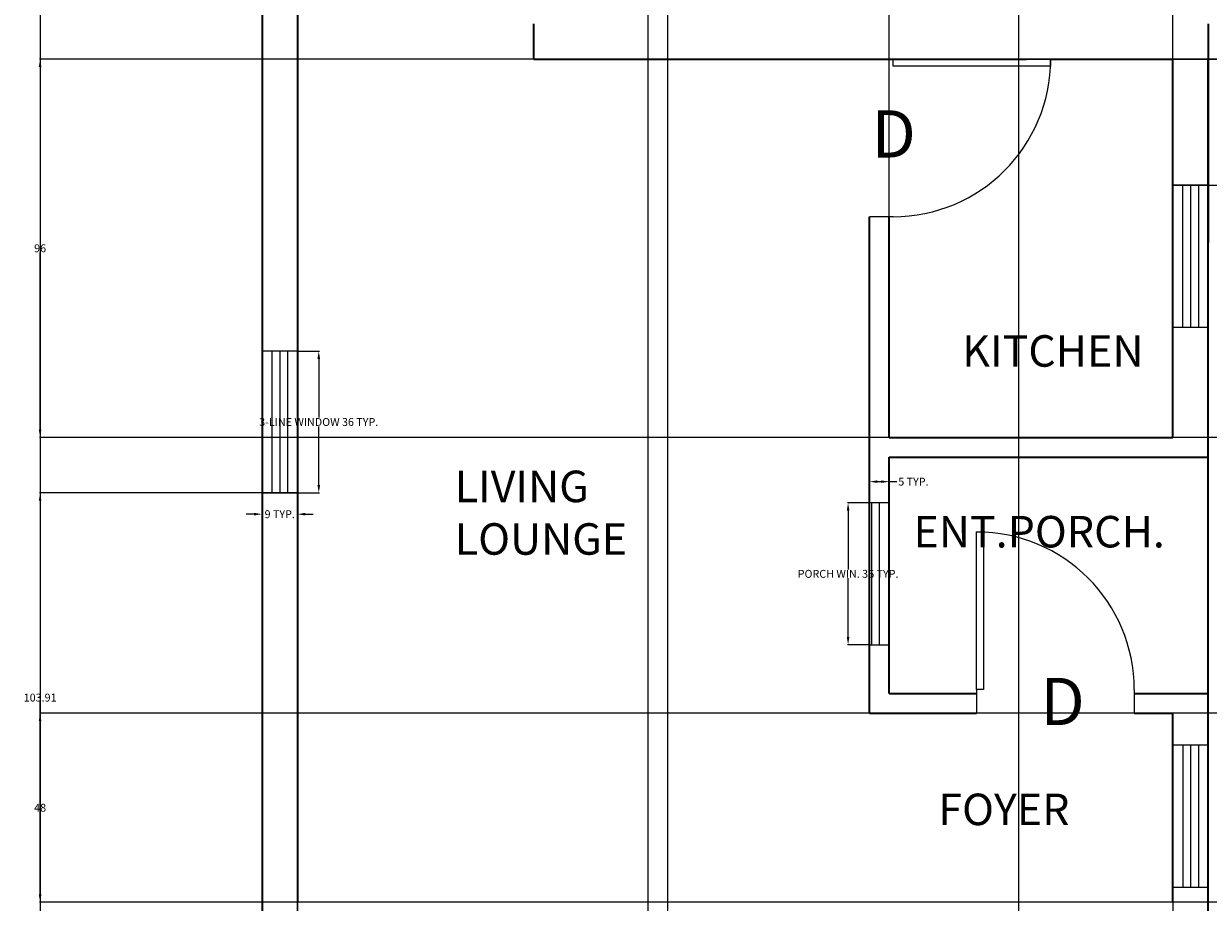
# Model space of a CAD drawing. Units: inches. Extents: x 190 to 836, y -241 to 999.
# Tile 6 of 9: x 190 to 491, y 566 to 789. Entities that reach past the tile are written whole.
import ezdxf

# ---------------------------------------------------------------- set-up
doc = ezdxf.new("R2010")
doc.units = ezdxf.units.IN
doc.header["$MEASUREMENT"] = 0
for name, color, linetype, lineweight in [('A-ANNO-DIMS', 2, 'Continuous', 18), ('A-ANNO-TEXT', 7, 'Continuous', 18), ('A-AREA-IDEN', 7, 'Continuous', 18), ('A-DOOR', 3, 'Continuous', 18), ('A-GLAZ', 4, 'Continuous', 18), ('A-WALL', 7, 'Continuous', 35)]:
    doc.layers.add(name, color=color, linetype=linetype, lineweight=lineweight)
doc.styles.get("Standard").update_dxf_attribs({"font": 'arial.ttf'})
doc.dimstyles.get("Standard").update_dxf_attribs({"dimtxt": 2, "dimasz": 2, "dimexe": 0.18, "dimexo": 0.0625, "dimgap": 0.09, "dimtad": 0, "dimtih": 1, "dimtoh": 1, "dimdec": 0, "dimzin": 0, "dimdsep": 46, "dimlunit": 3, "dimtxsty": 'Standard', "dimcen": 0.09, "dimadec": 0, "dimazin": 0, "dimtfac": 1, "dimtdec": 0, "dimtofl": 0, "dimtmove": 0, "dimatfit": 3, "dimfxl": 1, "dimtolj": 1, "dimtzin": 0, "dimarcsym": 0})

# ---------------------------------------------------------------- blocks, each defined once
blk = doc.blocks.new('*U4')
for p, q in [((-40, 0), (-40, 6)), ((0, 0), (0, 6))]:
    blk.add_line(p, q)
blk.add_lwpolyline([(0, 0), (0, -40), (-1.75, -40), (-1.75, 0)], close=True)
blk.add_arc((0, 0), 40, 180, 270)
blk = doc.blocks.new('*U5')
for p, q in [((0, 0), (0, -6)), ((40, 0), (40, -6))]:
    blk.add_line(p, q)
blk.add_lwpolyline([(0, 0), (0, 40), (1.75, 40), (1.75, 0)], close=True)
blk.add_arc((0, 0), 40, 0, 90)
blk = doc.blocks.new('WIN-36IN-9IN-3LINE')
for p, q in [((2.5, 36), (2.5, 0)), ((4.5, 36), (4.5, 0)), ((6.5, 36), (6.5, 0))]:
    blk.add_line(p, q)
blk.add_lwpolyline([(0, 0), (9, 0), (9, 36), (0, 36)], close=True)
blk = doc.blocks.new('WIN-36IN-5IN-PARTITION')
for p, q in [((5, 36), (0, 36)), ((0.5, 36), (0.5, 0)), ((2.5, 36), (2.5, 0)), ((5, 0), (5, 36)), ((0, 0), (5, 0))]:
    blk.add_line(p, q)
blk = doc.blocks.new('*D10')
at = {"layer": 'A-ANNO-DIMS', "color": 0, "lineweight": -2, "transparency": 16777216}
for p, q in [((259.5, 705.44), (265.02, 705.44)), ((264.84, 703.44), (264.84, 688.57)), ((264.84, 671.44), (264.84, 686.32)), ((259.5, 669.44), (265.02, 669.44))]:
    blk.add_line(p, q, dxfattribs=at)
at = {"layer": 'A-ANNO-DIMS', "color": 0, "transparency": 16777216}
for points in [[(264.51, 703.44), (265.18, 703.44), (264.84, 705.44)], [(264.51, 671.44), (265.18, 671.44), (264.84, 669.44)]]:
    blk.add_solid(points, dxfattribs=at)
at = {"layer": 'Defpoints', "color": 0, "transparency": 16777216}
for p in [(259.44, 705.44), (264.84, 705.44), (259.44, 669.44)]:
    blk.add_point(p, dxfattribs=at)
at = {"layer": 'A-ANNO-DIMS', "color": 0, "transparency": 16777216, "insert": (264.84, 687.44), "char_height": 2, "attachment_point": 5}
blk.add_mtext('\\A1;3-LINE WINDOW 36 TYP.', dxfattribs=at)
blk = doc.blocks.new('*D11')
at = {"layer": 'A-ANNO-DIMS', "color": 0, "lineweight": -2, "transparency": 16777216}
for p, q in [((250.44, 669.38), (250.44, 663.86)), ((259.44, 669.38), (259.44, 663.86)), ((248.44, 664.04), (246.44, 664.04)), ((261.44, 664.04), (263.44, 664.04))]:
    blk.add_line(p, q, dxfattribs=at)
at = {"layer": 'A-ANNO-DIMS', "color": 0, "transparency": 16777216}
for points in [[(248.44, 664.38), (248.44, 663.71), (250.44, 664.04)], [(261.44, 664.38), (261.44, 663.71), (259.44, 664.04)]]:
    blk.add_solid(points, dxfattribs=at)
at = {"layer": 'Defpoints', "color": 0, "transparency": 16777216}
for p in [(250.44, 669.44), (259.44, 669.44), (259.44, 664.04)]:
    blk.add_point(p, dxfattribs=at)
at = {"layer": 'A-ANNO-DIMS', "color": 0, "transparency": 16777216, "insert": (254.94, 664.04), "char_height": 2, "attachment_point": 5}
blk.add_mtext('\\A1;9 TYP.', dxfattribs=at)
blk = doc.blocks.new('*D14')
at = {"layer": 'A-ANNO-DIMS', "color": 0, "lineweight": -2, "transparency": 16777216}
for p, q in [((404.49, 666.9), (398.97, 666.9)), ((399.15, 664.9), (399.15, 650.03)), ((399.15, 632.9), (399.15, 647.77)), ((404.49, 630.9), (398.97, 630.9))]:
    blk.add_line(p, q, dxfattribs=at)
at = {"layer": 'A-ANNO-DIMS', "color": 0, "transparency": 16777216}
for points in [[(398.82, 664.9), (399.49, 664.9), (399.15, 666.9)], [(398.82, 632.9), (399.49, 632.9), (399.15, 630.9)]]:
    blk.add_solid(points, dxfattribs=at)
at = {"layer": 'Defpoints', "color": 0, "transparency": 16777216}
for p in [(399.15, 666.9), (404.55, 666.9), (404.55, 630.9)]:
    blk.add_point(p, dxfattribs=at)
at = {"layer": 'A-ANNO-DIMS', "color": 0, "transparency": 16777216, "insert": (399.15, 648.9), "char_height": 2, "attachment_point": 5}
blk.add_mtext('\\A1;PORCH WIN. 36 TYP.', dxfattribs=at)
blk = doc.blocks.new('*D15')
at = {"layer": 'A-ANNO-DIMS', "color": 0, "lineweight": -2, "transparency": 16777216}
for p, q in [((404.55, 666.96), (404.55, 672.48)), ((406.55, 672.3), (407.55, 672.3)), ((409.55, 666.96), (409.55, 672.48)), ((409.55, 672.3), (411.55, 672.3))]:
    blk.add_line(p, q, dxfattribs=at)
at = {"layer": 'A-ANNO-DIMS', "color": 0, "transparency": 16777216}
for points in [[(406.55, 672.63), (406.55, 671.97), (404.55, 672.3)], [(407.55, 672.63), (407.55, 671.97), (409.55, 672.3)]]:
    blk.add_solid(points, dxfattribs=at)
at = {"layer": 'Defpoints', "color": 0, "transparency": 16777216}
for p in [(409.55, 672.3), (404.55, 666.9), (409.55, 666.9)]:
    blk.add_point(p, dxfattribs=at)
at = {"layer": 'A-ANNO-DIMS', "color": 0, "transparency": 16777216, "insert": (415.73, 672.3), "char_height": 2, "attachment_point": 5}
blk.add_mtext('\\A1;5 TYP.', dxfattribs=at)
blk = doc.blocks.new('*D17')
at = {"layer": 'A-ANNO-DIMS', "color": 0, "lineweight": -2, "transparency": 16777216}
for p, q in [((250.38, 941.53), (193.96, 941.53)), ((194.14, 939.53), (194.14, 380.14)), ((194.14, -181.47), (194.14, 377.92)), ((447.38, -183.47), (193.96, -183.47))]:
    blk.add_line(p, q, dxfattribs=at)
at = {"layer": 'A-ANNO-DIMS', "color": 0, "transparency": 16777216}
for points in [[(193.8, 939.53), (194.47, 939.53), (194.14, 941.53)], [(193.8, -181.47), (194.47, -181.47), (194.14, -183.47)]]:
    blk.add_solid(points, dxfattribs=at)
at = {"layer": 'Defpoints', "color": 0, "transparency": 16777216}
for p in [(194.14, 941.53), (250.44, 941.53), (447.44, -183.47)]:
    blk.add_point(p, dxfattribs=at)
at = {"layer": 'A-ANNO-DIMS', "color": 0, "transparency": 16777216, "insert": (194.14, 379.03), "char_height": 2, "attachment_point": 5}
blk.add_mtext('\\A1;1125', dxfattribs=at)
blk = doc.blocks.new('*D26')
at = {"layer": 'A-ANNO-DIMS', "color": 0, "lineweight": -2, "transparency": 16777216}
for p, q in [((409.55, 683.59), (409.55, 998.02)), ((481.55, 683.59), (481.55, 998.02)), ((411.55, 997.84), (444.05, 997.84)), ((479.55, 997.84), (447.06, 997.84))]:
    blk.add_line(p, q, dxfattribs=at)
at = {"layer": 'A-ANNO-DIMS', "color": 0, "transparency": 16777216}
for points in [[(411.55, 998.17), (411.55, 997.5), (409.55, 997.84)], [(479.55, 998.17), (479.55, 997.5), (481.55, 997.84)]]:
    blk.add_solid(points, dxfattribs=at)
at = {"layer": 'Defpoints', "color": 0, "transparency": 16777216}
for p in [(481.55, 997.84), (409.55, 683.53), (481.55, 683.53)]:
    blk.add_point(p, dxfattribs=at)
at = {"layer": 'A-ANNO-DIMS', "color": 0, "transparency": 16777216, "insert": (445.55, 997.84), "char_height": 2, "attachment_point": 5}
blk.add_mtext('\\A1;72', dxfattribs=at)
blk = doc.blocks.new('*D27')
at = {"layer": 'A-ANNO-DIMS', "color": 0, "lineweight": -2, "transparency": 16777216}
for p, q in [((545.27, 779.53), (193.96, 779.53)), ((194.14, 777.53), (194.14, 732.64)), ((194.14, 685.53), (194.14, 730.42)), ((545.27, 683.53), (193.96, 683.53))]:
    blk.add_line(p, q, dxfattribs=at)
at = {"layer": 'A-ANNO-DIMS', "color": 0, "transparency": 16777216}
for points in [[(193.8, 777.53), (194.47, 777.53), (194.14, 779.53)], [(193.8, 685.53), (194.47, 685.53), (194.14, 683.53)]]:
    blk.add_solid(points, dxfattribs=at)
at = {"layer": 'Defpoints', "color": 0, "transparency": 16777216}
for p in [(194.14, 779.53), (545.33, 779.53), (545.33, 683.53)]:
    blk.add_point(p, dxfattribs=at)
at = {"layer": 'A-ANNO-DIMS', "color": 0, "transparency": 16777216, "insert": (194.14, 731.53), "char_height": 2, "attachment_point": 5}
blk.add_mtext('\\A1;96', dxfattribs=at)
blk = doc.blocks.new('*D29')
at = {"layer": 'A-ANNO-DIMS', "color": 0, "lineweight": -2, "transparency": 16777216}
for p, q in [((259.44, 565.47), (259.44, -239.95)), ((481.55, 565.47), (481.55, -239.95)), ((261.44, -239.77), (367.21, -239.77)), ((479.55, -239.77), (373.79, -239.77))]:
    blk.add_line(p, q, dxfattribs=at)
at = {"layer": 'A-ANNO-DIMS', "color": 0, "transparency": 16777216}
for points in [[(261.44, -239.44), (261.44, -240.11), (259.44, -239.77)], [(479.55, -239.44), (479.55, -240.11), (481.55, -239.77)]]:
    blk.add_solid(points, dxfattribs=at)
at = {"layer": 'Defpoints', "color": 0, "transparency": 16777216}
for p in [(259.44, 565.53), (481.55, 565.53), (481.55, -239.77)]:
    blk.add_point(p, dxfattribs=at)
at = {"layer": 'A-ANNO-DIMS', "color": 0, "transparency": 16777216, "insert": (370.5, -239.77), "char_height": 2, "attachment_point": 5}
blk.add_mtext('\\A1;222.1', dxfattribs=at)
blk = doc.blocks.new('*D30')
at = {"layer": 'A-ANNO-DIMS', "color": 0, "lineweight": -2, "transparency": 16777216}
for p, q in [((545.27, 613.53), (193.96, 613.53)), ((194.14, 611.53), (194.14, 590.64)), ((194.14, 567.53), (194.14, 588.42)), ((545.27, 565.53), (193.96, 565.53))]:
    blk.add_line(p, q, dxfattribs=at)
at = {"layer": 'A-ANNO-DIMS', "color": 0, "transparency": 16777216}
for points in [[(193.8, 611.53), (194.47, 611.53), (194.14, 613.53)], [(193.8, 567.53), (194.47, 567.53), (194.14, 565.53)]]:
    blk.add_solid(points, dxfattribs=at)
at = {"layer": 'Defpoints', "color": 0, "transparency": 16777216}
for p in [(194.14, 613.53), (545.33, 613.53), (545.33, 565.53)]:
    blk.add_point(p, dxfattribs=at)
at = {"layer": 'A-ANNO-DIMS', "color": 0, "transparency": 16777216, "insert": (194.14, 589.53), "char_height": 2, "attachment_point": 5}
blk.add_mtext('\\A1;48', dxfattribs=at)
blk = doc.blocks.new('*D35')
at = {"layer": 'A-ANNO-DIMS', "color": 0, "lineweight": -2, "transparency": 16777216}
for p, q in [((259.44, -8.41), (259.44, 998.02)), ((348.44, -8.41), (348.44, 998.02)), ((261.44, 997.84), (302.42, 997.84)), ((346.44, 997.84), (305.47, 997.84))]:
    blk.add_line(p, q, dxfattribs=at)
at = {"layer": 'A-ANNO-DIMS', "color": 0, "transparency": 16777216}
for points in [[(261.44, 998.17), (261.44, 997.5), (259.44, 997.84)], [(346.44, 998.17), (346.44, 997.5), (348.44, 997.84)]]:
    blk.add_solid(points, dxfattribs=at)
at = {"layer": 'Defpoints', "color": 0, "transparency": 16777216}
for p in [(348.44, 997.84), (259.44, -8.47), (348.44, -8.47)]:
    blk.add_point(p, dxfattribs=at)
at = {"layer": 'A-ANNO-DIMS', "color": 0, "transparency": 16777216, "insert": (303.94, 997.84), "char_height": 2, "attachment_point": 5}
blk.add_mtext('\\A1;89', dxfattribs=at)
blk = doc.blocks.new('*D36')
at = {"layer": 'A-ANNO-DIMS', "color": 0, "lineweight": -2, "transparency": 16777216}
for p, q in [((353.44, -8.41), (353.44, 998.02)), ((442.44, -8.41), (442.44, 998.02)), ((355.44, 997.84), (396.42, 997.84)), ((440.44, 997.84), (399.47, 997.84))]:
    blk.add_line(p, q, dxfattribs=at)
at = {"layer": 'A-ANNO-DIMS', "color": 0, "transparency": 16777216}
for points in [[(355.44, 998.17), (355.44, 997.5), (353.44, 997.84)], [(440.44, 998.17), (440.44, 997.5), (442.44, 997.84)]]:
    blk.add_solid(points, dxfattribs=at)
at = {"layer": 'Defpoints', "color": 0, "transparency": 16777216}
for p in [(442.44, 997.84), (353.44, -8.47), (442.44, -8.47)]:
    blk.add_point(p, dxfattribs=at)
at = {"layer": 'A-ANNO-DIMS', "color": 0, "transparency": 16777216, "insert": (397.94, 997.84), "char_height": 2, "attachment_point": 5}
blk.add_mtext('\\A1;89', dxfattribs=at)
blk = doc.blocks.new('*D51')
at = {"layer": 'A-ANNO-DIMS', "color": 0, "lineweight": -2, "transparency": 16777216}
for p, q in [((259.38, 669.44), (193.96, 669.44)), ((194.14, 667.44), (194.14, 618.6)), ((194.14, 567.53), (194.14, 616.38)), ((259.38, 565.53), (193.96, 565.53))]:
    blk.add_line(p, q, dxfattribs=at)
at = {"layer": 'A-ANNO-DIMS', "color": 0, "transparency": 16777216}
for points in [[(193.8, 667.44), (194.47, 667.44), (194.14, 669.44)], [(193.8, 567.53), (194.47, 567.53), (194.14, 565.53)]]:
    blk.add_solid(points, dxfattribs=at)
at = {"layer": 'Defpoints', "color": 0, "transparency": 16777216}
for p in [(194.14, 669.44), (259.44, 669.44), (259.44, 565.53)]:
    blk.add_point(p, dxfattribs=at)
at = {"layer": 'A-ANNO-DIMS', "color": 0, "transparency": 16777216, "insert": (194.14, 617.49), "char_height": 2, "attachment_point": 5}
blk.add_mtext('\\A1;103.91', dxfattribs=at)
blk = doc.blocks.new('*D53')
at = {"layer": 'A-ANNO-DIMS', "color": 0, "lineweight": -2, "transparency": 16777216}
for p, q in [((481.62, 779.53), (832.94, 779.53)), ((832.76, 777.53), (832.76, 764.64)), ((832.76, 749.53), (832.76, 762.42)), ((481.6, 747.53), (832.94, 747.53))]:
    blk.add_line(p, q, dxfattribs=at)
at = {"layer": 'A-ANNO-DIMS', "color": 0, "transparency": 16777216}
for points in [[(832.43, 777.53), (833.1, 777.53), (832.76, 779.53)], [(832.43, 749.53), (833.1, 749.53), (832.76, 747.53)]]:
    blk.add_solid(points, dxfattribs=at)
at = {"layer": 'Defpoints', "color": 0, "transparency": 16777216}
for p in [(481.55, 779.53), (832.76, 779.53), (481.54, 747.53)]:
    blk.add_point(p, dxfattribs=at)
at = {"layer": 'A-ANNO-DIMS', "color": 0, "transparency": 16777216, "insert": (832.76, 763.53), "char_height": 2, "attachment_point": 5}
blk.add_mtext('\\A1;32', dxfattribs=at)

msp = doc.modelspace()

# ---------------------------------------------------------------- linework, layer by layer
at = {"layer": 'A-WALL'}
for p, q in [((250.4421, 941.5313), (250.4421, 556.5313)), ((259.4421, 855.5313), (259.4421, 565.5313)), ((319.4421, 779.5313), (319.4421, 788.5313)), ((490.5536, 788.5313), (490.5536, 732.9119)), ((319.4421, 779.5313), (444.4421, 779.5313)), ((450.5536, 779.5313), (481.5536, 779.5313)), ((481.5536, 683.5313), (481.5536, 779.5313)), ((490.5536, 556.5313), (490.5536, 779.5313)), ((404.5536, 613.5313), (404.5536, 739.5313)), ((409.5536, 683.5313), (409.5536, 739.5313)), ((409.5536, 683.5313), (481.5536, 683.5313)), ((409.5536, 678.5313), (490.5536, 678.5313)), ((409.5536, 618.5313), (409.5536, 678.5313)), ((409.5536, 618.5313), (428.1141, 618.5313)), ((428.1141, 618.5313), (431.7728, 618.5313)), ((471.7728, 618.5313), (490.5536, 618.5313)), ((404.5536, 613.5313), (431.7728, 613.5313)), ((471.7728, 613.5313), (481.5536, 613.5313)), ((481.5536, 565.5313), (481.5536, 613.5313))]:
    msp.add_line(p, q, dxfattribs=at)

# ---------------------------------------------------------------- block references
at = {"layer": 'A-DOOR', "rotation": 90}
msp.add_blockref('*U4', (410.5536, 779.5313), dxfattribs=at)
at = {"layer": 'A-DOOR'}
msp.add_blockref('*U5', (431.7728, 619.5313), dxfattribs=at)
at = {"layer": 'A-GLAZ'}
for name, p in [('WIN-36IN-9IN-3LINE', (481.5422, 711.532)), ('WIN-36IN-9IN-3LINE', (250.442, 669.4424)), ('WIN-36IN-5IN-PARTITION', (404.554, 630.9)), ('WIN-36IN-9IN-3LINE', (481.5534, 569.3993))]:
    msp.add_blockref(name, p, dxfattribs=at)

# ---------------------------------------------------------------- texts
at = {"layer": 'A-ANNO-TEXT', "char_height": 12, "attachment_point": 1}
for insert in [(405.0847, 766.5566), (447.9408, 622.4981)]:
    msp.add_mtext_dynamic_manual_height_columns('D', width=8.765037, gutter_width=1, heights=[0], dxfattribs=dict(at, insert=insert))
at = {"layer": 'A-AREA-IDEN', "char_height": 8, "attachment_point": 1}
for s, insert in [('KITCHEN', (428.1017, 709.4705)), ('LIVING LOUNGE ', (299.3596, 675.086)), ('ENT.PORCH.', (415.7534, 663.5955)), ('FOYER', (422.0497, 593.1169))]:
    msp.add_mtext_dynamic_manual_height_columns(s, width=33.040256, gutter_width=1, heights=[0], dxfattribs=dict(at, insert=insert))

# ---------------------------------------------------------------- dimensions: what is measured, and where the dimension line sits
at = {"layer": 'A-ANNO-DIMS'}
for base, p1, p2, override, picture, middle in [((348.4421, 997.8363), (259.4421, -8.4687), (348.4421, -8.4687), {"dimdec": 0, "dimlfac": 1, "dimrnd": 0, "dimzin": 0, "dimdsep": 46, "dimlunit": 2}, '*D35', (303.9421, 997.8363)), ((442.4421, 997.8363), (353.4421, -8.4687), (442.4421, -8.4687), {"dimdec": 0, "dimlfac": 1, "dimrnd": 0, "dimzin": 0, "dimdsep": 46, "dimlunit": 2}, '*D36', (397.9421, 997.8363)), ((481.5536, 997.8363), (409.5536, 683.5313), (481.5536, 683.5313), {"dimdec": 0, "dimlfac": 1, "dimrnd": 0, "dimzin": 0, "dimdsep": 46, "dimlunit": 2}, '*D26', (445.5536, 997.8363)), ((481.5536, -239.7737), (259.4421, 565.5313), (481.5536, 565.5313), {"dimdec": 1, "dimlfac": 1, "dimrnd": 0, "dimzin": 0, "dimdsep": 46, "dimlunit": 2}, '*D29', (370.4979, -239.7737))]:
    dim = msp.add_linear_dim(base=base, p1=p1, p2=p2, dimstyle='Standard', override=override, dxfattribs=at)
    dim.commit()
    dim.dimension.update_dxf_attribs({"geometry": picture, "text_midpoint": middle})
for base, p1, p2, override, picture, middle in [((194.1371, 941.5313), (447.4421, -183.4687), (250.4421, 941.5313), {"dimdec": 0, "dimlfac": 1, "dimrnd": 0, "dimzin": 0, "dimdsep": 46, "dimlunit": 2}, '*D17', (194.1371, 379.0313)), ((194.1371, 779.5313), (545.3307, 683.5313), (545.3307, 779.5313), {"dimdec": 0, "dimlfac": 1, "dimrnd": 0, "dimzin": 0, "dimdsep": 46, "dimlunit": 2}, '*D27', (194.1371, 731.5313)), ((832.7634, 779.5313), (481.5423, 747.5319), (481.5536, 779.5313), {"dimdec": 0, "dimlfac": 1, "dimrnd": 0, "dimzin": 0, "dimdsep": 46, "dimlunit": 2}, '*D53', (832.7634, 763.5316)), ((194.1371, 669.4424), (259.4421, 565.5313), (259.4421, 669.4424), {"dimdec": 2, "dimlfac": 1, "dimrnd": 0, "dimzin": 0, "dimdsep": 46, "dimlunit": 2}, '*D51', (194.1371, 617.4869)), ((194.1371, 613.5313), (545.3307, 565.5313), (545.3307, 613.5313), {"dimdec": 0, "dimlfac": 1, "dimrnd": 0, "dimzin": 0, "dimdsep": 46, "dimlunit": 2}, '*D30', (194.1371, 589.5313))]:
    dim = msp.add_linear_dim(base=base, p1=p1, p2=p2, angle=90, dimstyle='Standard', override=override, dxfattribs=at)
    dim.commit()
    dim.dimension.update_dxf_attribs({"geometry": picture, "text_midpoint": middle})
for base, p1, p2, text, picture, middle in [((264.8421, 705.4424), (259.4421, 669.4424), (259.4421, 705.4424), '3-LINE WINDOW <> TYP.', '*D10', (264.8421, 687.4424)), ((399.1536, 666.9), (404.5536, 630.9), (404.5536, 666.9), 'PORCH WIN. <> TYP.', '*D14', (399.1536, 648.9))]:
    dim = msp.add_linear_dim(base=base, p1=p1, p2=p2, angle=90, text=text, dimstyle='Standard', override={"dimdec": 0, "dimlfac": 1, "dimrnd": 0, "dimzin": 0, "dimdsep": 46, "dimlunit": 2}, dxfattribs=at)
    dim.commit()
    dim.dimension.update_dxf_attribs({"geometry": picture, "text_midpoint": middle})
for base, p1, p2, picture, middle in [((409.5536, 672.3), (404.5536, 666.9), (409.5536, 666.9), '*D15', (415.7343, 672.3)), ((259.4421, 664.0424), (250.4421, 669.4424), (259.4421, 669.4424), '*D11', (254.9421, 664.0424))]:
    dim = msp.add_linear_dim(base=base, p1=p1, p2=p2, text='<> TYP.', dimstyle='Standard', override={"dimdec": 0, "dimlfac": 1, "dimrnd": 0, "dimzin": 0, "dimdsep": 46, "dimlunit": 2}, dxfattribs=at)
    dim.commit()
    dim.dimension.update_dxf_attribs({"geometry": picture, "text_midpoint": middle})

doc.saveas('drawing.dxf')
